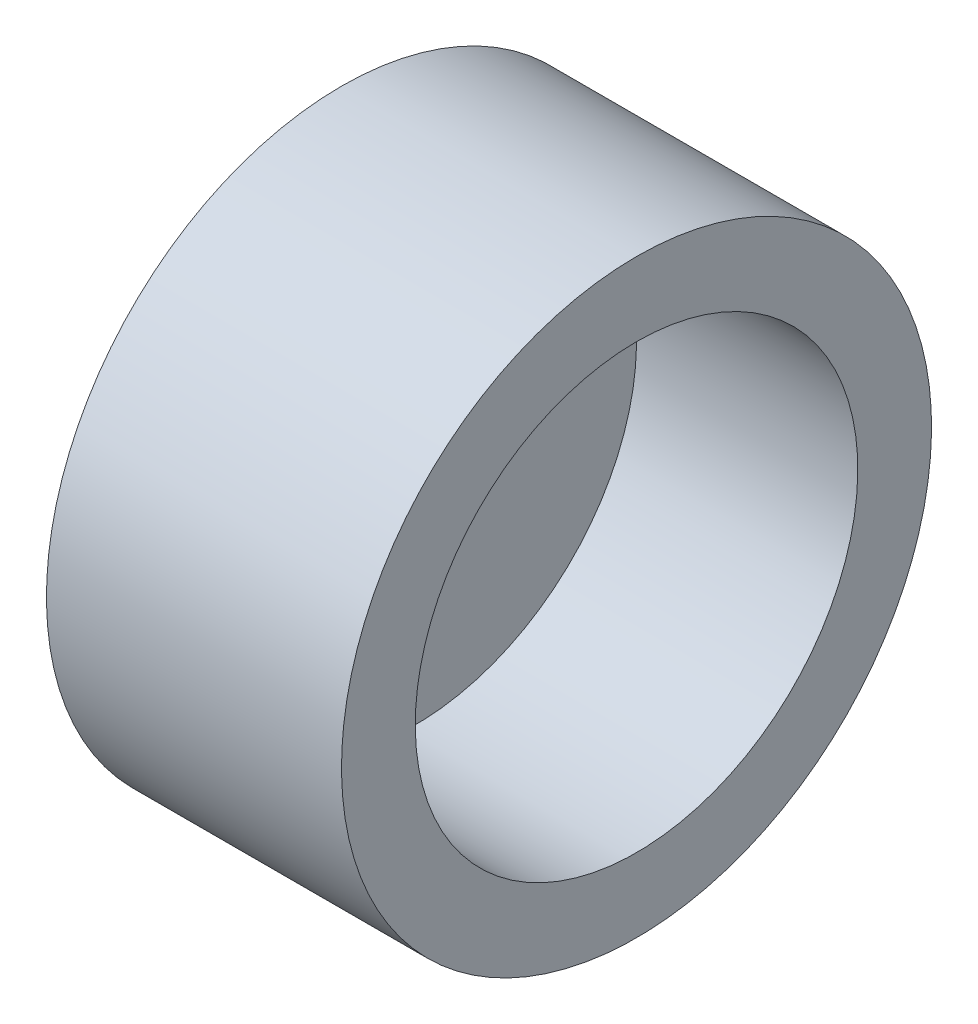
from build123d import *

# Parameters (mm, degrees)
COUNTERSUNK_CENTRE_HOLE_D                     = 6.858
COUNTERSUNK_CENTRE_HOLE_DEPTH                 = 19.05
COUNTERSUNK_CENTRE_HOLE_CSINK_D               = 13.208
COUNTERSUNK_CENTRE_HOLE_CSINK_ANGLE           = 82
COUNTERSUNK_CENTRE_HOLE_TIP                   = 2.060351063
COUNTERSUNK_CENTRE_HOLE_ON_FACE_2_D           = 6.858
COUNTERSUNK_CENTRE_HOLE_ON_FACE_2_DEPTH       = 19.05
COUNTERSUNK_CENTRE_HOLE_ON_FACE_2_CSINK_D     = 13.208
COUNTERSUNK_CENTRE_HOLE_ON_FACE_2_CSINK_ANGLE = 82
COUNTERSUNK_CENTRE_HOLE_ON_FACE_2_TIP         = 2.060351063


with BuildPart() as part:
    # Cup Profile Sketch → Cup Body Revolve (revolve)
    with BuildSketch(Plane.XY):
        Polygon((-19.05, 0), (-25.4, 0), (-25.4, 25.4), (0, 25.4), (0, 19.05), (-19.05, 19.05), align=None)
    revolve(axis=Axis((-19.05, 0, 0), (-1, 0, 0)))

    # Countersunk Centre Hole
    with Locations(Plane(origin=(-25.4, 0, 0), x_dir=(0, -1, 0), z_dir=(-1, 0, 0))):
        with Locations((0, 0)):
            CounterSinkHole(COUNTERSUNK_CENTRE_HOLE_D / 2, COUNTERSUNK_CENTRE_HOLE_CSINK_D / 2, depth=COUNTERSUNK_CENTRE_HOLE_DEPTH, counter_sink_angle=COUNTERSUNK_CENTRE_HOLE_CSINK_ANGLE)
            with Locations((0, 0, -(COUNTERSUNK_CENTRE_HOLE_DEPTH + COUNTERSUNK_CENTRE_HOLE_TIP / 2))):  # 118° drill point
                Cone(0, COUNTERSUNK_CENTRE_HOLE_D / 2, COUNTERSUNK_CENTRE_HOLE_TIP, mode=Mode.SUBTRACT)

    # Countersunk Centre Hole on face 2
    with Locations(Plane(origin=(0, 0, 0), x_dir=(0, -1, 0), z_dir=(-1, 0, 0))):
        with Locations((0, 0)):
            CounterSinkHole(COUNTERSUNK_CENTRE_HOLE_ON_FACE_2_D / 2, COUNTERSUNK_CENTRE_HOLE_ON_FACE_2_CSINK_D / 2, depth=COUNTERSUNK_CENTRE_HOLE_ON_FACE_2_DEPTH, counter_sink_angle=COUNTERSUNK_CENTRE_HOLE_ON_FACE_2_CSINK_ANGLE)
            with Locations((0, 0, -(COUNTERSUNK_CENTRE_HOLE_ON_FACE_2_DEPTH + COUNTERSUNK_CENTRE_HOLE_ON_FACE_2_TIP / 2))):  # 118° drill point
                Cone(0, COUNTERSUNK_CENTRE_HOLE_ON_FACE_2_D / 2, COUNTERSUNK_CENTRE_HOLE_ON_FACE_2_TIP, mode=Mode.SUBTRACT)


solid = part.part
